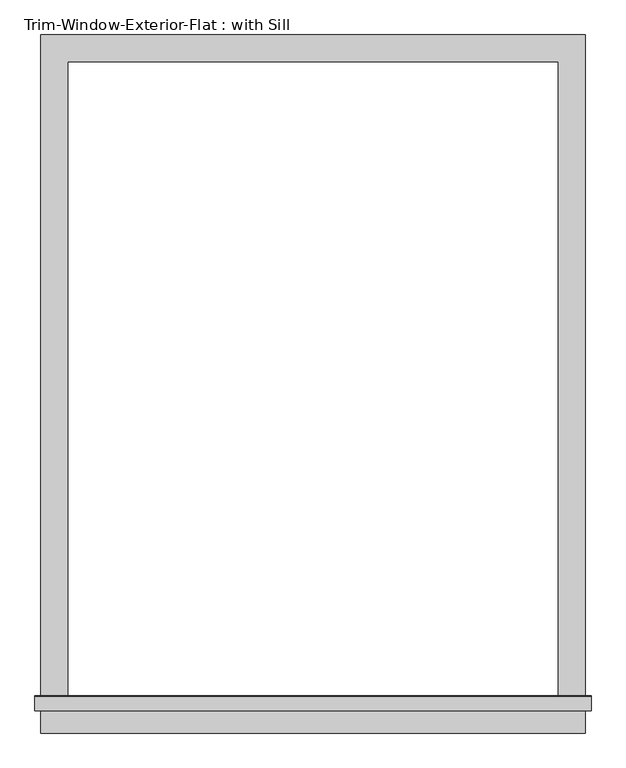
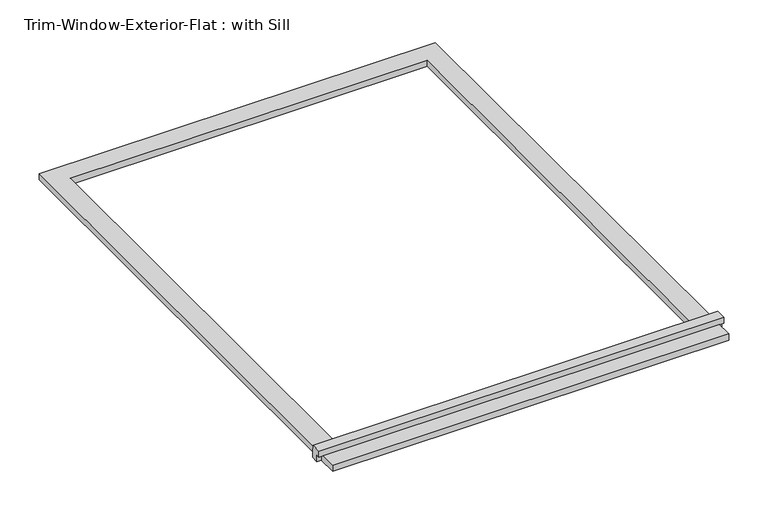
"""IFC4 building model written with IfcOpenShell, lengths in millimetres: proxy geometry, Trim-Window-Exterior-Flat : with Sill."""

from ifc_helpers import new_model, si_unit, frame, origin, origin_with_axes, place, context, project, spatial, polyline, outline, extrude, source, transform, mapped, element, save


def trim_window_exterior_flat_with_sill_4930676f(model_context):
    return source(origin(), model_context, "Body", "SweptSolid", [
        extrude(outline(polyline([(577.85, -1368.3823709), (577.85, -1425.5323709), (-577.85, -1425.5323709), (-577.85, -1368.3823709), (577.85, -1368.3823709)])), origin_with_axes(), (0.0, 0.0, 1.0), 19.05),
        extrude(outline(polyline([(-1377.95, 38.1), (-1348.6580645, 38.1), (-1346.2, 19.05), (-1346.2, 0.0), (-1368.3823709, 0.0), (-1368.3823709, 19.05), (-1377.95, 19.05), (-1377.95, 38.1)])), frame((-590.55, 0.0, 0.0), z_axis=(1.0, 0.0, 0.0), x_axis=(0.0, 1.0, 0.0)), (0.0, 0.0, 1.0), 1181.1),
        extrude(outline(polyline([(-577.85, 57.15), (577.85, 57.15), (577.85, -1346.2), (520.7, -1346.2), (520.7, 0.0), (-520.7, 0.0), (-520.7, -1346.2), (-577.85, -1346.2), (-577.85, 57.15)])), origin_with_axes(), (0.0, 0.0, 1.0), 19.05),
    ])


if __name__ == "__main__":
    model = new_model("IFC4")
    model_context = context("Model", 3, world=origin())
    ifc_project = project(units=[si_unit("LENGTHUNIT", "METRE", prefix="MILLI")], contexts=[model_context])
    site = spatial("IfcSite", under=ifc_project)
    building = spatial("IfcBuilding", under=site)
    placement = place(None, origin())
    trim_window_exterior_flat_with_sill_shape = trim_window_exterior_flat_with_sill_4930676f(model_context)
    element("IfcBuildingElementProxy", 1, Name="Trim-Window-Exterior-Flat : with Sill", ObjectType="Trim-Window-Exterior-Flat : with Sill", at=placement, inside=building, context=model_context, shape_type="MappedRepresentation", body=[
        mapped(trim_window_exterior_flat_with_sill_shape, transform((0.0, 0.0, 0.0), x_axis=(1.0, 0.0, 0.0), y_axis=(0.0, 1.0, 0.0), z_axis=(0.0, 0.0, 1.0))),
    ])
    save(model, "model.ifc")

# Revit data of these elements
# Type "Trim-Window-Exterior-Flat : with Sill"
#   Trim Width = 0' - 2 1/4"
#   Trim Thickness_Picture Frame = 0' - 1 1/4"
#   Trim Thickness_with Sill = 0' - 0 3/4"
#   Sill Thickness = 0' - 1 1/4"
#   Opening Width [instance default] = 2' - 0"
#   Opening Height [instance default] = 3' - 0"
#   Default Elevation = 4' - 0"
#   Sill = yes
#   Picture Frame = no
#   Trim Material [instance default] = none
# Element 1 (IfcBuildingElementProxy, "Trim-Window-Exterior-Flat : with Sill")
#   Opening Width = 3' - 5"
#   Opening Height = 4' - 5"
#   Trim Material = Clad - White
#   Materials on its faces: "Clad - White"
# Materials
#   "Clad - White": class "Wood", colour RGB 242 242 238, transparency 0, Cost = 0
